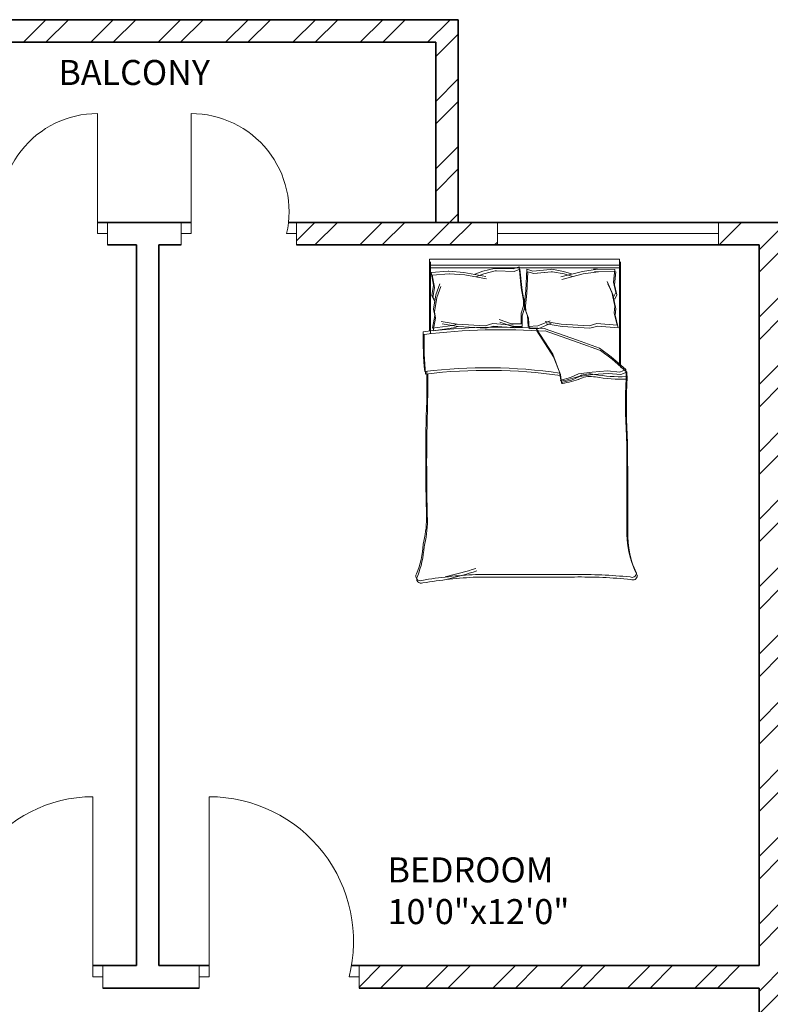
# Model space of a CAD drawing. Units: inches. Extents: x 1944 to 3454, y 1352 to 3055.
# Tile 7 of 17: x 2163 to 2314, y 2026 to 2223. Entities that reach past the tile are written whole.
import ezdxf

# ---------------------------------------------------------------- set-up
doc = ezdxf.new("R2010")
doc.units = ezdxf.units.IN
for name, color, linetype, lineweight in [('A-AREA-IDEN', 7, 'Continuous', 18), ('A-DOOR', 3, 'Continuous', 20), ('A-FURN', 8, 'Continuous', 13), ('A-GLAZ', 4, 'Continuous', 18), ('A-WALL', 7, 'Continuous', 35), ('A-WALL-PATT', 252, 'Continuous', 13)]:
    doc.layers.add(name, color=color, linetype=linetype, lineweight=lineweight)
doc.styles.get("Standard").update_dxf_attribs({"font": 'arial.ttf'})

# ---------------------------------------------------------------- blocks, each defined once
blk = doc.blocks.new('BED-WITH-PILLOWS-01')
for p, q in [((22.05, 42.02), (19.47, 39.08)), ((22.05, 42.02), (19.47, 39.08)), ((22.56, 42.21), (19.98, 39.26)), ((22.56, 42.21), (19.98, 39.26)), ((23.44, 42.09), (22.05, 42.02, 3.08)), ((23.44, 42.09), (22.05, 42.02, 3.08)), ((22.55, 40.8), (22.05, 42.02)), ((22.55, 40.8), (22.05, 42.02)), ((23.95, 42.27), (22.56, 42.21, 3.08)), ((23.95, 42.27), (22.56, 42.21, 3.08)), ((23.05, 40.98), (22.56, 42.21)), ((23.05, 40.98), (22.56, 42.21)), ((0, 40.75), (21.15, 40.75)), ((0, 40.75), (21.15, 40.75)), ((0, 2.76), (0, 40.75)), ((0.51, 40.93), (21.66, 40.93)), ((0.51, 40.93), (21.66, 40.93)), ((1.22, 2.76), (1.22, 40.75)), ((1.22, 2.76), (1.22, 40.75)), ((1.73, 2.94), (1.73, 40.93)), ((1.73, 2.94), (1.73, 40.93)), ((2.03, 39.83), (1.96, 35.54)), ((2.03, 39.83), (1.96, 35.54)), ((2.03, 39.83), (4.58, 39.53)), ((2.03, 39.83), (4.58, 39.53)), ((2.54, 40.01), (2.46, 35.72)), ((2.54, 40.01), (2.46, 35.72)), ((2.54, 40.01), (5.09, 39.71)), ((2.54, 40.01), (5.09, 39.71)), ((4.58, 39.53), (6.63, 40.01)), ((4.58, 39.53), (6.63, 40.01)), ((7.07, 39.38), (4.94, 38.44)), ((7.07, 39.38), (4.94, 38.44)), ((5.09, 39.71), (7.14, 40.19)), ((5.09, 39.71), (7.14, 40.19)), ((9.4, 39.83), (6.56, 39.2)), ((9.4, 39.83), (6.56, 39.2)), ((6.63, 40.01), (7.46, 39.6)), ((6.63, 40.01), (7.46, 39.6)), ((9.91, 40.01), (7.07, 39.38)), ((9.91, 40.01), (7.07, 39.38)), ((7.14, 40.19), (7.97, 39.78)), ((7.14, 40.19), (7.97, 39.78)), ((10.68, 39.68), (9.4, 39.83)), ((10.68, 39.68), (9.4, 39.83)), ((11.19, 39.86), (9.91, 40.01)), ((11.19, 39.86), (9.91, 40.01)), ((13.17, 40.3), (10.68, 39.68)), ((13.17, 40.3), (10.68, 39.68)), ((13.68, 40.48), (11.19, 39.86)), ((13.68, 40.48), (11.19, 39.86)), ((12.85, 36.22), (13.17, 40.3)), ((12.85, 36.22), (13.17, 40.3)), ((13.36, 36.4), (13.68, 40.48)), ((13.36, 36.4), (13.68, 40.48)), ((22.3, 38.34), (22.55, 40.8)), ((22.3, 38.34), (22.55, 40.8)), ((22.81, 38.52), (23.05, 40.98)), ((22.81, 38.52), (23.05, 40.98)), ((6.56, 39.2), (4.43, 38.26)), ((6.56, 39.2), (4.43, 38.26)), ((19.47, 39.08), (17.75, 36.74)), ((19.47, 39.08), (17.75, 36.74)), ((19.98, 39.26), (18.26, 36.92)), ((19.98, 39.26), (18.26, 36.92)), ((22.55, 35.26), (22.3, 38.34)), ((22.55, 35.26), (22.3, 38.34)), ((23.05, 35.44), (22.81, 38.52)), ((23.05, 35.44), (22.81, 38.52)), ((1.96, 35.54), (2.02, 36.34)), ((1.96, 35.54), (2.02, 36.34)), ((2.02, 36.34), (2.44, 33.32)), ((2.02, 36.34), (2.44, 33.32)), ((2.46, 35.72), (2.53, 36.52)), ((2.46, 35.72), (2.53, 36.52)), ((2.53, 36.52), (2.95, 33.5)), ((2.53, 36.52), (2.95, 33.5)), ((13.3, 34.66), (12.85, 36.22)), ((13.3, 34.66), (12.85, 36.22)), ((13.8, 34.84), (13.36, 36.4)), ((13.8, 34.84), (13.36, 36.4)), ((17.75, 36.74), (16.15, 32.31)), ((17.75, 36.74), (16.15, 32.31)), ((18.26, 36.92), (16.66, 32.49)), ((18.26, 36.92), (16.66, 32.49)), ((23.42, 32.74), (23.05, 35.44)), ((23.42, 32.74), (23.05, 35.44)), ((2.95, 33.5), (4.02, 29.19)), ((2.95, 33.5), (4.02, 29.19)), ((12.95, 29.09), (13.3, 34.66)), ((12.95, 29.09), (13.3, 34.66)), ((13.46, 29.27), (13.8, 34.84)), ((13.46, 29.27), (13.8, 34.84)), ((22.92, 32.55), (22.55, 35.26)), ((22.92, 32.55), (22.55, 35.26)), ((2.44, 33.32), (3.51, 29.01)), ((2.44, 33.32), (3.51, 29.01)), ((16.15, 32.31), (13.82, 25.68)), ((16.15, 32.31), (13.82, 25.68)), ((16.66, 32.49), (14.33, 25.86)), ((16.66, 32.49), (14.33, 25.86)), ((23.65, 30.95), (22.92, 32.55)), ((23.65, 30.95), (22.92, 32.55)), ((24.16, 31.13), (23.42, 32.74)), ((24.16, 31.13), (23.42, 32.74)), ((62.99, 11.97), (62.99, 31.54)), ((62.99, 11.97), (62.99, 31.54)), ((63.5, 12.16), (63.5, 31.72)), ((63.5, 12.15), (63.5, 31.72)), ((2.45, 29.52), (2.02, 27.19)), ((2.45, 29.52), (2.02, 27.19)), ((2.92, 31.16), (2.45, 29.52)), ((2.92, 31.16), (2.45, 29.52)), ((2.95, 29.7), (2.52, 27.37)), ((2.95, 29.7), (2.52, 27.37)), ((3.43, 31.34), (2.95, 29.7)), ((3.43, 31.34), (2.95, 29.7)), ((24.15, 28.98), (23.65, 30.95)), ((24.15, 28.98), (23.65, 30.95)), ((24.65, 29.17), (24.16, 31.13)), ((24.65, 29.16), (24.16, 31.13)), ((12.42, 25.88), (12.95, 29.09)), ((12.42, 25.88), (12.95, 29.09)), ((12.93, 26.07), (13.46, 29.27)), ((12.93, 26.07), (13.46, 29.27)), ((14.33, 24.23), (19.49, 27.56)), ((14.33, 24.23), (19.49, 27.56)), ((18.98, 27.38), (22.55, 28.74)), ((18.98, 27.38), (22.55, 28.74)), ((19.49, 27.56), (23.05, 28.92)), ((19.49, 27.56), (23.05, 28.92)), ((22.55, 28.74), (24.15, 28.98)), ((22.55, 28.74), (24.15, 28.98)), ((23.05, 28.92), (24.65, 29.17)), ((23.05, 28.92), (24.65, 29.16)), ((2.02, 27.19), (2.03, 26.93)), ((2.02, 27.19), (2.03, 26.93)), ((2.03, 26.93), (2.37, 23.41)), ((2.03, 26.93), (2.37, 23.41)), ((2.52, 27.37), (2.54, 27.12)), ((2.52, 27.37), (2.54, 27.11)), ((2.54, 27.12), (2.88, 23.6)), ((2.54, 27.11), (2.88, 23.6)), ((13.31, 24.44), (12.28, 26.88)), ((13.31, 24.44), (12.28, 26.88)), ((13.81, 24.62), (12.79, 27.07)), ((13.81, 24.62), (12.79, 27.06)), ((13.82, 24.05), (18.98, 27.38)), ((13.82, 24.05), (18.98, 27.38)), ((13.43, 22.49), (13.31, 24.44)), ((13.43, 22.49), (13.31, 24.44)), ((13.94, 22.67), (13.81, 24.62)), ((13.94, 22.67), (13.81, 24.62)), ((2.37, 23.41), (1.98, 22.24)), ((2.37, 23.41), (1.98, 22.24)), ((1.98, 22.24), (6.25, 22.04)), ((1.98, 22.24), (6.25, 22.04)), ((2.88, 23.6), (2.49, 22.42)), ((2.88, 23.6), (2.49, 22.42)), ((2.49, 22.42), (6.76, 22.23)), ((2.49, 22.42), (6.76, 22.23)), ((6.25, 22.04), (8.81, 21.74)), ((6.25, 22.04), (8.81, 21.74)), ((6.25, 21.29), (8.78, 21.75)), ((6.25, 21.29), (8.78, 21.75)), ((6.76, 22.23), (9.31, 21.93)), ((6.76, 22.23), (9.31, 21.93)), ((8.78, 21.75), (9.81, 21.75)), ((8.78, 21.75), (9.81, 21.75)), ((8.81, 21.74), (9.84, 21.81)), ((8.81, 21.74), (9.84, 21.81)), ((9.31, 21.93), (10.35, 21.99)), ((9.31, 21.93), (10.35, 21.99)), ((9.81, 21.75), (11.3, 21.29)), ((9.81, 21.75), (11.3, 21.29)), ((9.84, 21.81), (11.3, 22.36)), ((9.84, 21.81), (11.3, 22.36)), ((10.35, 21.99), (11.81, 22.54)), ((10.35, 21.99), (11.81, 22.54)), ((11.3, 22.36), (13.43, 22.49)), ((11.3, 22.36), (13.43, 22.49)), ((11.81, 22.54), (13.94, 22.67)), ((11.81, 22.54), (13.94, 22.67)), ((1.49, 20.65), (5.74, 21.11)), ((1.49, 20.65), (5.74, 21.11)), ((1.95, 19.5), (1.49, 20.65)), ((1.95, 19.5), (1.49, 20.65)), ((1.99, 20.83), (6.25, 21.29)), ((1.99, 20.83), (6.25, 21.29)), ((2.45, 19.69), (1.99, 20.83)), ((2.45, 19.69), (1.99, 20.83)), ((2.34, 16.15), (2.45, 19.69)), ((2.34, 16.15), (2.45, 19.69)), ((5.74, 21.11), (8.27, 21.57)), ((5.74, 21.11), (8.27, 21.57)), ((8.27, 21.57), (9.3, 21.57)), ((8.27, 21.57), (9.3, 21.57)), ((9.3, 21.57), (10.8, 21.11)), ((9.3, 21.57), (10.8, 21.11)), ((10.8, 21.11), (12.93, 21.11)), ((10.8, 21.11), (12.93, 21.11)), ((11.3, 21.29), (13.44, 21.29)), ((11.3, 21.29), (13.44, 21.29)), ((12.93, 21.11), (12.93, 19.16)), ((12.93, 21.11), (12.93, 19.16)), ((13.44, 21.29), (13.44, 19.34)), ((13.44, 21.29), (13.44, 19.34)), ((1.83, 15.97), (1.95, 19.5)), ((1.83, 15.97), (1.95, 19.5)), ((12.93, 19.16), (12.06, 16.66)), ((12.93, 19.16), (12.06, 16.66)), ((13.44, 19.34), (12.57, 16.84)), ((13.44, 19.34), (12.57, 16.84)), ((12.85, 15.41), (13.17, 19.49)), ((12.85, 15.41), (13.17, 19.49)), ((13.36, 15.59), (13.68, 19.67)), ((13.36, 15.59), (13.68, 19.67)), ((1.83, 15.71), (1.83, 15.97)), ((1.83, 15.71), (1.83, 15.97)), ((2.34, 15.9), (2.34, 16.15)), ((2.34, 15.9), (2.34, 16.15)), ((2.91, 13.6), (2.34, 15.9)), ((2.91, 13.6), (2.34, 15.9)), ((2.41, 13.42), (1.83, 15.71)), ((2.41, 13.42), (1.83, 15.71)), ((2.64, 9.62), (3.44, 13.99)), ((2.64, 9.62), (3.44, 13.99)), ((3.14, 9.81), (3.95, 14.17)), ((3.14, 9.81), (3.95, 14.17)), ((13.3, 13.85), (12.85, 15.41)), ((13.3, 13.85), (12.85, 15.41)), ((12.95, 8.28), (13.3, 13.85)), ((12.95, 8.28), (13.3, 13.85)), ((13.8, 14.03), (13.36, 15.59)), ((13.8, 14.03), (13.36, 15.59)), ((13.46, 8.46), (13.8, 14.03)), ((13.46, 8.46), (13.8, 14.03)), ((2.98, 11.81), (2.41, 13.42)), ((2.98, 11.81), (2.41, 13.42)), ((3.49, 11.99), (2.91, 13.6)), ((3.49, 11.99), (2.91, 13.6)), ((2.41, 6.59), (2.64, 9.62)), ((2.41, 6.59), (2.64, 9.62)), ((2.91, 6.77), (3.14, 9.81)), ((2.91, 6.77), (3.14, 9.81)), ((12.42, 5.07), (12.95, 8.28)), ((12.42, 5.07), (12.95, 8.28)), ((12.93, 5.25), (13.46, 8.46)), ((12.93, 5.25), (13.46, 8.46)), ((12.95, 8.28), (13.21, 7.38)), ((12.95, 8.28), (13.21, 7.38)), ((13.46, 8.46), (13.72, 7.56)), ((13.46, 8.46), (13.72, 7.56)), ((2.39, 6.5), (2.41, 6.59)), ((2.39, 6.5), (2.41, 6.59)), ((2.65, 3.1), (2.39, 6.5)), ((2.65, 3.1), (2.39, 6.5)), ((2.9, 6.68), (2.91, 6.77)), ((2.9, 6.68), (2.91, 6.77)), ((3.16, 3.28), (2.9, 6.68)), ((3.16, 3.28), (2.9, 6.68)), ((13.21, 7.38), (13.78, 3.33)), ((13.21, 7.38), (13.78, 3.33)), ((13.72, 7.56), (14.29, 3.51)), ((13.72, 7.56), (14.29, 3.51)), ((7.12, 4.02), (4.93, 4.82)), ((7.12, 4.01), (4.93, 4.82)), ((7.63, 4.2), (5.44, 5)), ((7.63, 4.2), (5.44, 5)), ((9.99, 3.56), (7.12, 4.02)), ((9.99, 3.56), (7.12, 4.01)), ((10.5, 3.74), (7.63, 4.2)), ((10.5, 3.74), (7.63, 4.2)), ((11.76, 3.97), (10.5, 3.74)), ((11.76, 3.97), (10.5, 3.74)), ((14.29, 3.51), (11.76, 3.97)), ((14.29, 3.51), (11.76, 3.97)), ((14.4, 2.76), (0, 2.76)), ((14.4, 2.76), (0, 2.76)), ((14.9, 2.94), (0.51, 2.94)), ((14.9, 2.94), (0.51, 2.94)), ((2.64, 3.1), (5.16, 3.56)), ((2.64, 3.1), (5.16, 3.56)), ((3.14, 3.28), (5.67, 3.74)), ((3.14, 3.28), (5.67, 3.74)), ((5.16, 3.56), (7.23, 3.21)), ((5.16, 3.56), (7.23, 3.21)), ((5.67, 3.74), (7.74, 3.39)), ((5.67, 3.74), (7.74, 3.39)), ((7.23, 3.21), (8.04, 3.67)), ((7.23, 3.21), (8.04, 3.67)), ((7.74, 3.39), (8.55, 3.85)), ((7.74, 3.39), (8.55, 3.85)), ((11.26, 3.79), (9.99, 3.56)), ((11.26, 3.79), (9.99, 3.56)), ((13.78, 3.33), (11.26, 3.79)), ((13.78, 3.33), (11.26, 3.79))]:
    blk.add_line(p, q)
for centre, radius, start, end in [((54.58, 60.54), 18.33, 267.4714, 296.4681), ((54.58, 60.54), 18.33, 267.4714, 296.4681), ((55.09, 60.72), 18.33, 267.4714, 296.4681), ((55.09, 60.72), 18.33, 267.4714, 296.4681), ((62.69, 43.25), 0.876, 332.6588, 86.02), ((62.69, 43.25), 0.876, 332.6588, 86.02), ((63.2, 43.43), 0.876, 332.6588, 86.02), ((63.2, 43.43), 0.876, 332.6588, 86.02), ((-5.29, 40.8), 28.76, 349.8763, 2.5657), ((-5.29, 40.8), 28.76, 349.8763, 2.5657), ((28.87, 144.88), 102.94, 266.9791, 273.8365), ((28.87, 144.88), 102.94, 266.9791, 273.8365), ((-4.78, 40.98), 28.76, 349.8763, 2.5657), ((-4.78, 40.98), 28.76, 349.8763, 2.5657), ((29.37, 145.06), 102.94, 266.9791, 273.8365), ((29.37, 145.06), 102.94, 266.9791, 273.8365), ((53.91, -3583.94), 3626.16, 90.00217, 90.28689), ((53.91, -3583.94), 3626.16, 90.00217, 90.28689), ((54.42, -3583.76), 3626.16, 90.00217, 90.28689), ((54.42, -3583.76), 3626.16, 90.00217, 90.28689), ((168.74, 32.71), 105.75, 174.4998, 180.6351), ((168.74, 32.71), 105.75, 174.4998, 180.6351), ((169.24, 32.89), 105.75, 174.4998, 180.6351), ((169.24, 32.89), 105.75, 174.4998, 180.6351), ((27.87, 34.77), 4.95, 168.6608, 203.7384), ((27.87, 34.77), 4.95, 168.6608, 203.7384), ((28.38, 34.95), 4.95, 168.6608, 203.7384), ((28.38, 34.95), 4.95, 168.6608, 203.7384), ((1.18, 24.76), 23.57, 10.6617, 19.8806), ((1.18, 24.76), 23.57, 10.6617, 19.8806), ((1.69, 24.95), 23.57, 10.6617, 19.8806), ((1.69, 24.94), 23.57, 10.6617, 19.8806), ((124.25, 14.11), 102.56, 171.7845, 186.9006), ((124.25, 14.11), 102.56, 171.7845, 186.9006), ((124.76, 14.3), 102.56, 171.7845, 186.9006), ((124.76, 14.3), 102.56, 171.7845, 186.9006), ((24.2, 29.12), 0.147, 250.2464, 1.1377), ((24.2, 29.12), 0.147, 250.2464, 1.1377), ((24.7, 29.3), 0.147, 250.2464, 1.1377), ((24.7, 29.3), 0.147, 250.2464, 1.1377), ((144.71, 16.98), 131.13, 176.0865, 186.7821), ((144.71, 16.98), 131.13, 176.0865, 186.7821), ((145.22, 17.16), 131.13, 176.0865, 186.7821), ((145.22, 17.16), 131.13, 176.0865, 186.7821), ((-18.85, -13.69), 84.62, 13.3832, 17.7053), ((-18.85, -13.69), 84.62, 13.3832, 17.7053), ((-18.34, -13.51), 84.62, 13.3832, 17.7053), ((-18.34, -13.51), 84.62, 13.3832, 17.7053), ((159.64, 17.03), 96.78, 182.9958, 189.4091), ((159.64, 17.03), 96.78, 182.9958, 189.4091), ((160.15, 17.21), 96.78, 182.9958, 189.4091), ((160.15, 17.21), 96.78, 182.9958, 189.4091), ((16.48, 67.88), 66.22, 268.7218, 275.604), ((16.48, 67.88), 66.22, 268.7218, 275.604), ((24.78, -132.99), 135.22, 88.4762, 91.0082), ((24.78, -132.99), 135.22, 88.4762, 91.0082), ((25.29, -132.81), 135.22, 88.4762, 91.0082), ((25.29, -132.81), 135.22, 88.4762, 91.0082), ((40.23, 385.38), 383.38, 268.2277, 271.7185), ((40.23, 385.38), 383.38, 268.2277, 271.7185), ((40.74, 385.56), 383.38, 268.2277, 271.7185), ((40.74, 385.56), 383.38, 268.2277, 271.7185), ((51.28, -21.38), 23.56, 76.0648, 88.9113), ((51.28, -21.38), 23.56, 76.0648, 88.9113), ((51.79, -21.2), 23.56, 76.0648, 88.9113), ((51.79, -21.2), 23.56, 76.0648, 88.9113), ((15.97, 67.69), 66.22, 268.7218, 275.604), ((15.97, 67.69), 66.22, 268.7218, 275.604), ((55.86, -17.22), 18.73, 67.9751, 86.652), ((55.86, -17.22), 18.73, 67.9751, 86.652), ((56.37, -17.04), 18.73, 67.9751, 86.652), ((56.37, -17.04), 18.73, 67.9751, 86.652), ((63.37, 0.86), 0.866, 236.1736, 23.4781), ((63.37, 0.86), 0.866, 236.1736, 23.4781), ((63.87, 1.05), 0.866, 236.1736, 23.4781), ((63.87, 1.05), 0.866, 236.1736, 23.4781)]:
    blk.add_arc(centre, radius, start, end)
blk = doc.blocks.new('DOOR-SWING-36IN-03')
for p, q in [((2, 2.25), (2, 38.25)), ((0, 4.5), (0, 0)), ((32, 4.5), (32, 0)), ((0, 0), (0, 2.25)), ((0, 2.25), (2, 2.25)), ((32, 2.25), (30, 2.25)), ((32, 0), (32, 2.25))]:
    blk.add_line(p, q)
blk.add_arc((2, 9.36), 28.89, 345.7565, 90)
blk = doc.blocks.new('DOOR-SWING-36IN-04')
for p, q in [((27.8, 2.25), (27.8, 38.25)), ((0, 0), (0, 4.5)), ((29.8, 4.5), (29.8, 0)), ((0, 2.25), (2, 2.25)), ((29.8, 2.25), (27.8, 2.25)), ((29.8, 0), (29.8, 2.25))]:
    blk.add_line(p, q)
blk.add_arc((27.8, 11), 27.25, 90, 198.7358)
blk = doc.blocks.new('DOOR-SWING-24IN-01')
for p, q in [((20.84, 2.25), (20.84, 26.25)), ((0, 4.5), (0, 0)), ((22.84, 0), (22.84, 4.5)), ((22.84, 4.5), (22.84, 2.25)), ((0, 0), (0, 2.25)), ((0, 2.25), (2, 2.25)), ((22.84, 2.25), (20.84, 2.25))]:
    blk.add_line(p, q)
blk.add_arc((20.84, 6.85), 19.4, 90, 193.7219)
blk = doc.blocks.new('DOOR-SWING-24IN-02')
for p, q in [((2, 2.25), (2, 26.25)), ((0, 0), (0, 4.5)), ((0, 4.5), (0, 2.25)), ((23.1, 4.5), (23.1, 0)), ((0, 2.25), (2, 2.25)), ((23.1, 2.25), (21.1, 2.25)), ((23.1, 0), (23.1, 2.25))]:
    blk.add_line(p, q)
blk.add_arc((2, 6.65), 19.6, 347.0256, 90)
blk = doc.blocks.new('WINDOW-PLAN-44.19IN-01')
for p, q in [((0, 4.5), (0, 0)), ((44.19, 2.25), (44.19, 4.5)), ((44.19, 4.5), (44.19, 0)), ((0, 0), (0, 2.25)), ((0, 2.25), (44.19, 2.25))]:
    blk.add_line(p, q)

msp = doc.modelspace()

# ---------------------------------------------------------------- hatches: boundary and pattern name
at = {"layer": 'A-WALL-PATT'}
h = msp.add_hatch(dxfattribs=at)
h.set_pattern_fill('ANSI32', color=256)
h.paths.add_polyline_path([(2061.822, 2177.596), (2158.181, 2177.596), (2158.181, 2179.846), (2158.181, 2182.096), (2057.322, 2182.096), (2057.322, 2123.452), (2061.822, 2123.452)])
h.paths.add_polyline_path([(2258.993, 2179.846), (2258.993, 2182.096), (2218.838, 2182.096), (2218.838, 2177.596), (2258.993, 2177.596)])
h.paths.add_polyline_path([(2315.822, 2177.596), (2322.722, 2177.596), (2322.722, 2182.096), (2303.186, 2182.096), (2303.186, 2177.596), (2311.322, 2177.596), (2311.322, 2033.596), (2231.355, 2033.596), (2231.355, 2029.096), (2311.322, 2029.096), (2311.322, 1904.596), (2307.941, 1904.596), (2307.941, 1900.096), (2319.277, 1900.096), (2319.277, 1902.346), (2319.277, 1904.596), (2315.822, 1904.596), (2315.822, 2029.096), (2394.855, 2029.096), (2394.855, 2033.596), (2315.822, 2033.596)])
h.paths.add_polyline_path([(2407.334, 2182.096), (2366.1, 2182.096), (2366.1, 2177.596), (2407.334, 2177.596), (2407.334, 2179.846)])
h.paths.add_polyline_path([(2440.322, 2177.596), (2443.866, 2177.596), (2443.866, 2182.096), (2431.827, 2182.096), (2431.827, 2179.846), (2431.827, 2177.596), (2435.822, 2177.596), (2435.822, 2033.596), (2430.464, 2033.596), (2430.464, 2029.096), (2445.372, 2029.096), (2445.372, 2031.346), (2445.372, 2033.596), (2440.322, 2033.596)])
h.paths.add_polyline_path([(2569.822, 2182.096), (2466.481, 2182.096), (2466.481, 2177.596), (2565.322, 2177.596), (2565.322, 2123.452), (2569.822, 2123.452)])
h.paths.add_polyline_path([(2569.822, 2063.452), (2567.572, 2063.452), (2565.322, 2063.452), (2565.322, 2033.596), (2478.08, 2033.596), (2476.822, 2033.596), (2476.822, 2028.698), (2476.822, 2020.069), (2481.322, 2020.069), (2481.322, 2029.096), (2565.322, 2029.096), (2565.322, 2014.5), (2569.822, 2014.5)])
h.paths.add_polyline_path([(2569.822, 1978.5), (2565.322, 1978.5), (2565.322, 1957.096), (2481.322, 1957.096), (2481.322, 1990.369), (2476.822, 1990.369), (2476.822, 1957.096), (2476.822, 1952.596), (2476.822, 1947.471), (2481.322, 1947.471), (2481.322, 1952.596), (2565.322, 1952.596), (2565.322, 1943.2), (2569.822, 1943.2)])
h.paths.add_polyline_path([(2569.822, 1919.2), (2565.322, 1919.2), (2565.322, 1904.596), (2481.322, 1904.596), (2481.322, 1928.596), (2476.822, 1928.596), (2476.822, 1904.596), (2350.518, 1904.596), (2350.518, 1900.096), (2476.822, 1900.096), (2565.322, 1900.096), (2565.322, 1895.596), (2565.322, 1887.047), (2569.822, 1887.047)])
h.paths.add_polyline_path([(2280.492, 1904.596), (2150.322, 1904.596), (2150.322, 1926.68), (2148.072, 1926.68), (2145.822, 1926.68), (2145.822, 1904.596), (2061.822, 1904.596), (2061.822, 1914.977), (2059.572, 1914.977), (2057.322, 1914.977), (2057.322, 1887.362), (2061.822, 1887.362), (2061.822, 1900.096), (2150.322, 1900.096), (2280.492, 1900.096), (2280.492, 1902.346)])
h.paths.add_polyline_path([(2150.322, 1957.096), (2150.322, 1986.22), (2145.822, 1986.22), (2145.822, 1957.096), (2061.822, 1957.096), (2061.822, 1975.678), (2057.322, 1975.678), (2057.322, 1938.977), (2061.822, 1938.977), (2061.822, 1952.596), (2145.822, 1952.596), (2145.822, 1947.985), (2150.322, 1947.985), (2150.322, 1952.596)])
h.paths.add_polyline_path([(2061.822, 2063.452), (2057.322, 2063.452), (2057.322, 2011.678), (2061.822, 2011.678), (2061.822, 2029.096), (2145.288, 2029.096), (2145.822, 2029.096), (2145.822, 2019.118), (2150.322, 2019.118), (2150.322, 2029.096), (2150.322, 2033.596), (2147.022, 2033.596), (2061.822, 2033.596)])
h.paths.add_polyline_path([(2061.822, 1835.596), (2133.822, 1835.596), (2133.822, 1794.415), (2138.322, 1794.415), (2138.322, 1835.596), (2231.726, 1835.596), (2231.726, 1840.096), (2061.822, 1840.096), (2061.822, 1851.362), (2057.322, 1851.362), (2057.322, 1810.528), (2061.822, 1810.528)])
h.paths.add_polyline_path([(2061.822, 1774.528), (2059.572, 1774.528), (2057.322, 1774.528), (2057.322, 1723.746), (2061.822, 1723.746), (2061.822, 1735.096), (2133.822, 1735.096), (2133.822, 1731.415), (2138.322, 1731.415), (2138.322, 1759.737), (2133.822, 1759.737), (2133.822, 1739.596), (2061.822, 1739.596)])
h.paths.add_polyline_path([(2061.822, 1678.596), (2147.597, 1678.596), (2147.597, 1680.846), (2147.597, 1683.096), (2138.322, 1683.096), (2138.322, 1710.66), (2136.072, 1710.66), (2133.822, 1710.66), (2133.822, 1683.096), (2061.822, 1683.096), (2061.822, 1699.746), (2057.322, 1699.746), (2057.322, 1645.751), (2061.822, 1645.751)])
h.paths.add_polyline_path([(2061.822, 1585.751), (2057.322, 1585.751), (2057.322, 1530.096), (2158.703, 1530.096), (2158.703, 1534.596), (2061.822, 1534.596)])
h.paths.add_polyline_path([(2191.322, 1678.596), (2195.889, 1678.596), (2195.889, 1683.096), (2181.763, 1683.096), (2181.763, 1680.846), (2181.763, 1678.596), (2186.822, 1678.596), (2186.822, 1534.596), (2181.354, 1534.596), (2181.354, 1530.096), (2196.54, 1530.096), (2196.54, 1532.346), (2196.54, 1534.596), (2191.322, 1534.596)])
h.paths.add_polyline_path([(2315.822, 1678.596), (2402.014, 1678.596), (2402.014, 1683.096), (2355.822, 1683.096), (2355.822, 1835.596), (2360.838, 1835.596), (2360.838, 1840.096), (2351.322, 1840.096), (2351.322, 1683.096), (2273.322, 1683.096), (2273.322, 1840.096), (2263.134, 1840.096), (2263.134, 1837.846), (2263.134, 1835.596), (2268.822, 1835.596), (2268.822, 1683.096), (2227.793, 1683.096), (2227.793, 1678.596), (2311.322, 1678.596), (2311.322, 1534.596), (2302.384, 1534.596), (2302.384, 1530.096), (2324.521, 1530.096), (2324.521, 1532.346), (2324.521, 1534.596), (2315.822, 1534.596)])
h.paths.add_polyline_path([(2440.322, 1678.596), (2443.656, 1678.596), (2443.656, 1683.096), (2432.614, 1683.096), (2432.614, 1680.846), (2432.614, 1678.596), (2435.822, 1678.596), (2435.822, 1534.596), (2440.322, 1534.596)])
h.paths.add_polyline_path([(2409.913, 1534.596), (2369.033, 1534.596), (2369.033, 1530.096), (2409.913, 1530.096)])
h.paths.add_polyline_path([(2259.529, 1532.346), (2259.529, 1534.596), (2218.889, 1534.596), (2218.889, 1532.346), (2218.889, 1530.096), (2259.529, 1530.096)])
h.paths.add_polyline_path([(2569.822, 1584.389), (2567.572, 1584.389), (2565.322, 1584.389), (2565.322, 1534.596), (2465.892, 1534.596), (2465.892, 1530.096), (2569.822, 1530.096)])
h.paths.add_polyline_path([(2505.567, 1530.096), (2501.067, 1530.096), (2501.067, 1494.096), (2381.067, 1494.096), (2381.067, 1530.096), (2376.567, 1530.096), (2376.567, 1489.596), (2381.067, 1489.596), (2505.567, 1489.596), (2505.567, 1494.096)])
h.paths.add_polyline_path([(2127.673, 1530.096), (2123.173, 1530.096), (2123.173, 1489.596), (2127.673, 1489.596), (2252.173, 1489.596), (2252.173, 1494.096), (2252.173, 1530.096), (2247.673, 1530.096), (2247.673, 1494.096), (2127.673, 1494.096)])
h.paths.add_polyline_path([(2251.167, 2222.596), (2126.667, 2222.596), (2122.167, 2222.596), (2122.167, 2182.096), (2126.667, 2182.096), (2126.667, 2218.096), (2210.667, 2218.096), (2234.667, 2218.096), (2246.667, 2218.096), (2246.667, 2182.096), (2251.167, 2182.096), (2251.167, 2218.096)])
h.paths.add_polyline_path([(2501.916, 2222.596), (2497.416, 2222.596), (2372.916, 2222.596), (2372.916, 2218.096), (2372.916, 2182.096), (2377.416, 2182.096), (2377.416, 2218.096), (2497.416, 2218.096), (2497.416, 2182.096), (2501.916, 2182.096)])
h.paths.add_polyline_path([(2569.822, 1700.442), (2565.322, 1700.442), (2565.322, 1683.096), (2493.322, 1683.096), (2493.322, 1709.096), (2488.822, 1709.096), (2488.822, 1683.096), (2475.416, 1683.096), (2475.416, 1680.846), (2475.416, 1678.596), (2488.822, 1678.596), (2565.322, 1678.596), (2565.322, 1644.389), (2569.822, 1644.389)])
h.paths.add_polyline_path([(2569.822, 1773.506), (2565.322, 1773.506), (2565.322, 1739.596), (2493.322, 1739.596), (2493.322, 1754.002), (2488.822, 1754.002), (2488.822, 1729.846), (2491.072, 1729.846), (2493.322, 1729.846), (2493.322, 1735.096), (2565.322, 1735.096), (2565.322, 1724.442), (2569.822, 1724.442)])
h.paths.add_polyline_path([(2569.822, 1851.047), (2567.572, 1851.047), (2565.322, 1851.047), (2565.322, 1840.096), (2395.039, 1840.096), (2395.039, 1837.846), (2395.039, 1835.596), (2488.822, 1835.596), (2488.822, 1798.423), (2493.322, 1798.423), (2493.322, 1835.596), (2565.322, 1835.596), (2565.322, 1809.506), (2569.822, 1809.506)])
h.paths.add_polyline_path([(2347.275, 1955.576), (2414.024, 1955.576), (2414.024, 1974.234), (2347.275, 1974.234)], flags=9)
h.paths.add_polyline_path([(2509.756, 1990.497), (2542.915, 1990.497), (2542.915, 2009.154), (2509.756, 2009.154)], flags=9)

# ---------------------------------------------------------------- linework, layer by layer
at = {"layer": 'A-WALL'}
for p, q in [((2251.167, 2222.596), (2126.667, 2222.596)), ((2251.167, 2218.096), (2251.167, 2222.596)), ((2126.667, 2218.096), (2210.667, 2218.096)), ((2210.667, 2218.096), (2234.667, 2218.096)), ((2234.667, 2218.096), (2246.667, 2218.096)), ((2246.667, 2218.096), (2246.667, 2182.096)), ((2251.167, 2182.096), (2251.167, 2218.096)), ((2179.025, 2182.096), (2197.738, 2182.096)), ((2217.22, 2182.096), (2409.102, 2182.096)), ((2246.667, 2182.096), (2251.167, 2182.096)), ((2181.025, 2177.596), (2186.822, 2177.596)), ((2186.822, 2177.596), (2186.822, 2033.596)), ((2191.322, 2177.596), (2191.322, 2033.596)), ((2191.322, 2177.596), (2195.738, 2177.596)), ((2218.838, 2177.596), (2311.322, 2177.596)), ((2311.322, 2177.596), (2311.322, 2033.596)), ((2178.126, 2033.596), (2186.822, 2033.596)), ((2191.322, 2033.596), (2201.351, 2033.596)), ((2229.831, 2033.596), (2311.322, 2033.596)), ((2180.126, 2029.096), (2199.351, 2029.096)), ((2231.355, 2029.096), (2311.322, 2029.096)), ((2311.322, 2029.096), (2311.322, 1904.596))]:
    msp.add_line(p, q, dxfattribs=at)

# ---------------------------------------------------------------- block references
at = {"layer": 'A-DOOR'}
for name, p in [('DOOR-SWING-24IN-01', (2158.181, 2177.596)), ('DOOR-SWING-24IN-02', (2195.738, 2177.596)), ('DOOR-SWING-36IN-04', (2150.322, 2029.096)), ('DOOR-SWING-36IN-03', (2199.351, 2029.096))]:
    msp.add_blockref(name, p, dxfattribs=at)
at = {"layer": 'A-FURN', "rotation": 270}
msp.add_blockref('BED-WITH-PILLOWS-01', (2242.67, 2174.739), dxfattribs=at)
at = {"layer": 'A-GLAZ'}
msp.add_blockref('WINDOW-PLAN-44.19IN-01', (2258.993, 2177.596), dxfattribs=at)

# ---------------------------------------------------------------- texts
at = {"layer": 'A-AREA-IDEN', "char_height": 5, "attachment_point": 1}
for s, width, insert in [('BALCONY', 118.50767, (2171.217, 2214.553)), ('BEDROOM\\P10\'0"x12\'0"', 131.85907, (2237.029, 2055.229))]:
    msp.add_mtext_dynamic_manual_height_columns(s, width=width, gutter_width=12.5, heights=[0], dxfattribs=dict(at, insert=insert))

doc.saveas('drawing.dxf')
